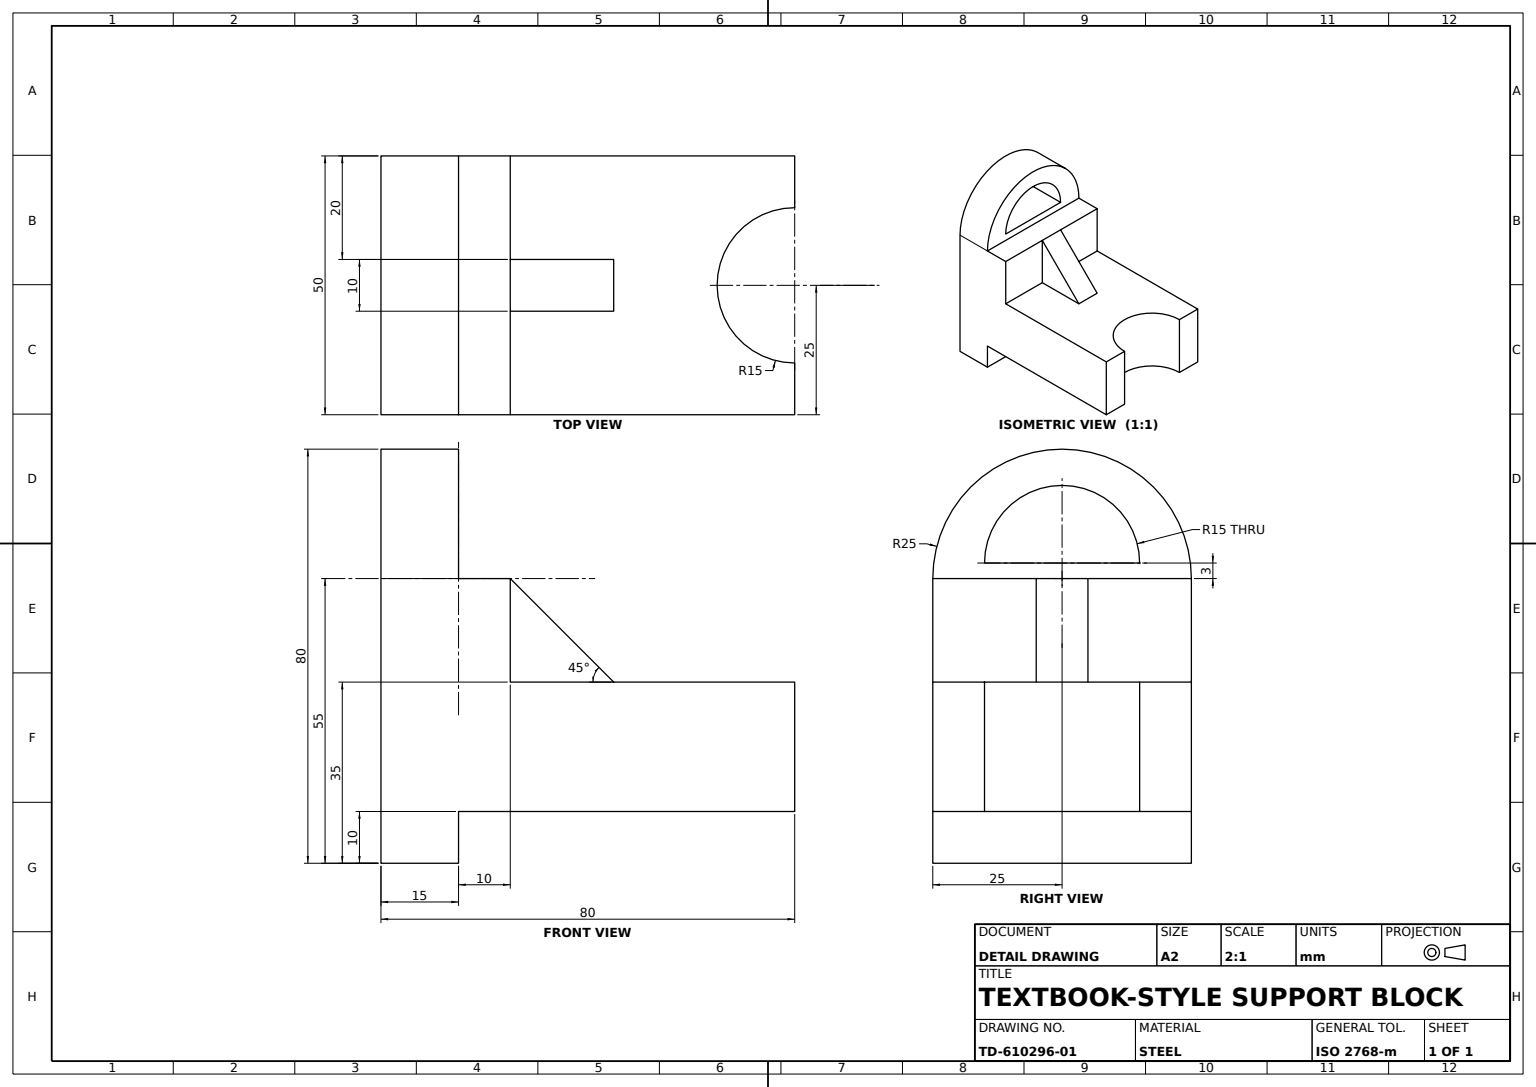
SolidWorks part; units mm, degrees
material "Plain Carbon Steel"
ref_plane "Front Plane" through (0, 0, 0) normal (0, 0, 1) x (1, 0, 0)
ref_plane "Top Plane" through (0, 0, 0) normal (0, 1, 0) x (1, 0, 0)
ref_plane "Right Plane" through (0, 0, 0) normal (1, 0, 0) x (0, 0, -1)
sketch "Base Profile Sketch" plane through (0, 0, 0) normal (0, 0, 1) x (1, 0, 0)
  line L0 (0, 0) -> (0, 55)
  line L1 (0, 55) -> (10, 55)
  line L2 (10, 55) -> (10, 35)
  line L3 (10, 35) -> (75, 35)
  line L4 (75, 35) -> (75, 10)
  line L5 (75, 10) -> (10, 10)
  line L6 (10, 10) -> (10, 0)
  line L7 (10, 0) -> (0, 0)
  dimension "D1" = 10
  dimension "D2" = 75
  dimension "D3" = 35
  dimension "D4" = 55
extrude "Base Block 50mm" add sketch "Base Profile Sketch" along normal blind 50
sketch "Step Boss Sketch" plane through (0, 0, 0) normal (-1, 0, 0) x (0, 0, 1)
  line L0 (0, 55) -> (50, 55)
  line L1 (50, 55) -> (50, 0)
  line L2 (50, 0) -> (0, 0)
  line L3 (0, 0) -> (0, 55)
extrude "Step Boss 10mm" add sketch "Step Boss Sketch" along normal blind 10
sketch "Step Cut Sketch" plane through (-10, 0, 0) normal (-1, 0, 0) x (0, 0, 1)
  line L0 (0, 55) -> (50, 55)
  line L1 (50, 55) -> (50, 0)
  line L2 (50, 0) -> (0, 0)
  line L3 (0, 0) -> (0, 55)
extrude "Step Cut 10mm" cut sketch "Step Cut Sketch" against normal blind 10
sketch "Upright Pad Sketch" plane through (0, 0, 0) normal (-1, 0, 0) x (0, 0, 1)
  line L0 (0, 55) -> (50, 55)
  line L1 (50, 55) -> (50, 0)
  line L2 (50, 0) -> (0, 0)
  line L3 (0, 0) -> (0, 55)
extrude "Upright Pad 5mm" add sketch "Upright Pad Sketch" along normal blind 5
sketch "Arch Boss Sketch R25" plane through (-5, 0, 0) normal (-1, 0, 0) x (0, 0, 1)
  line L0 (50, 55) -> (0, 55) construction
  line L1 (0, 55) -> (50, 55)
  arc A0 (50, 55) -> (0, 55) centre (25, 55) ccw
  dimension "D1" = 50
extrude "Arch Boss 15mm" add sketch "Arch Boss Sketch R25" against normal blind 15
sketch "Upper Block Sketch" plane through (10, 0, 0) normal (1, 0, 0) x (0, 0, -1)
  line L0 (-50, 35) -> (-50, 55)
  line L1 (-50, 55) -> (0, 55)
  line L2 (0, 55) -> (0, 35)
  line L3 (0, 35) -> (-50, 35)
extrude "Upper Block 10mm" add sketch "Upper Block Sketch" along normal blind 10
sketch "Base Notch Sketch Ø30" plane through (10, 0, 0) normal (1, 0, 0) x (0, 0, -1)
  line L0 (0, 55) -> (-50, 55) construction
  line L2 (-25, 58) -> (-10, 58)
  line L3 (-10, 58) -> (-40, 58)
  arc A0 (-10, 58) -> (-40, 58) centre (-25, 58) ccw
  dimension "D1" = 30
  dimension "D2" = 15
  dimension "D3" = 25
  dimension "D4" = 3
extrude "Base Semicircular Notch" cut sketch "Base Notch Sketch Ø30" against normal blind 15 contours L2 A0 L3
sketch "Arch Cut Sketch Ø30" plane through (0, 35, 0) normal (0, 1, 0) x (1, 0, 0)
  line L0 (75, -50) -> (75, 0) construction
  line L1 (75, -10) -> (75, -40)
  arc A0 (75, -10) -> (75, -40) centre (75, -25) ccw
  dimension "D1" = 30
  dimension "D2" = 15
extrude "Arch Semicircular Cut" cut sketch "Arch Cut Sketch Ø30" against normal blind 25
sketch "Rib Sketch" plane through (0, 0, 50) normal (0, 0, 1) x (1, 0, 0)
  line L0 (20, 55) -> (20, 35)
  line L1 (20, 35) -> (40, 35)
  line L2 (75, 35) -> (20, 35) construction
  line L3 (40, 35) -> (20, 55)
extrude "Support Rib 30mm" add sketch "Rib Sketch" against normal blind 30
sketch "Rib Trim Sketch" plane through (0, 0, 50) normal (0, 0, 1) x (1, 0, 0)
  line L0 (20, 55) -> (20, 35)
  line L1 (20, 35) -> (40, 35)
  line L2 (40, 35) -> (20, 55)
extrude "Rib Trim Cut 20mm" cut sketch "Rib Trim Sketch" against normal blind 20
